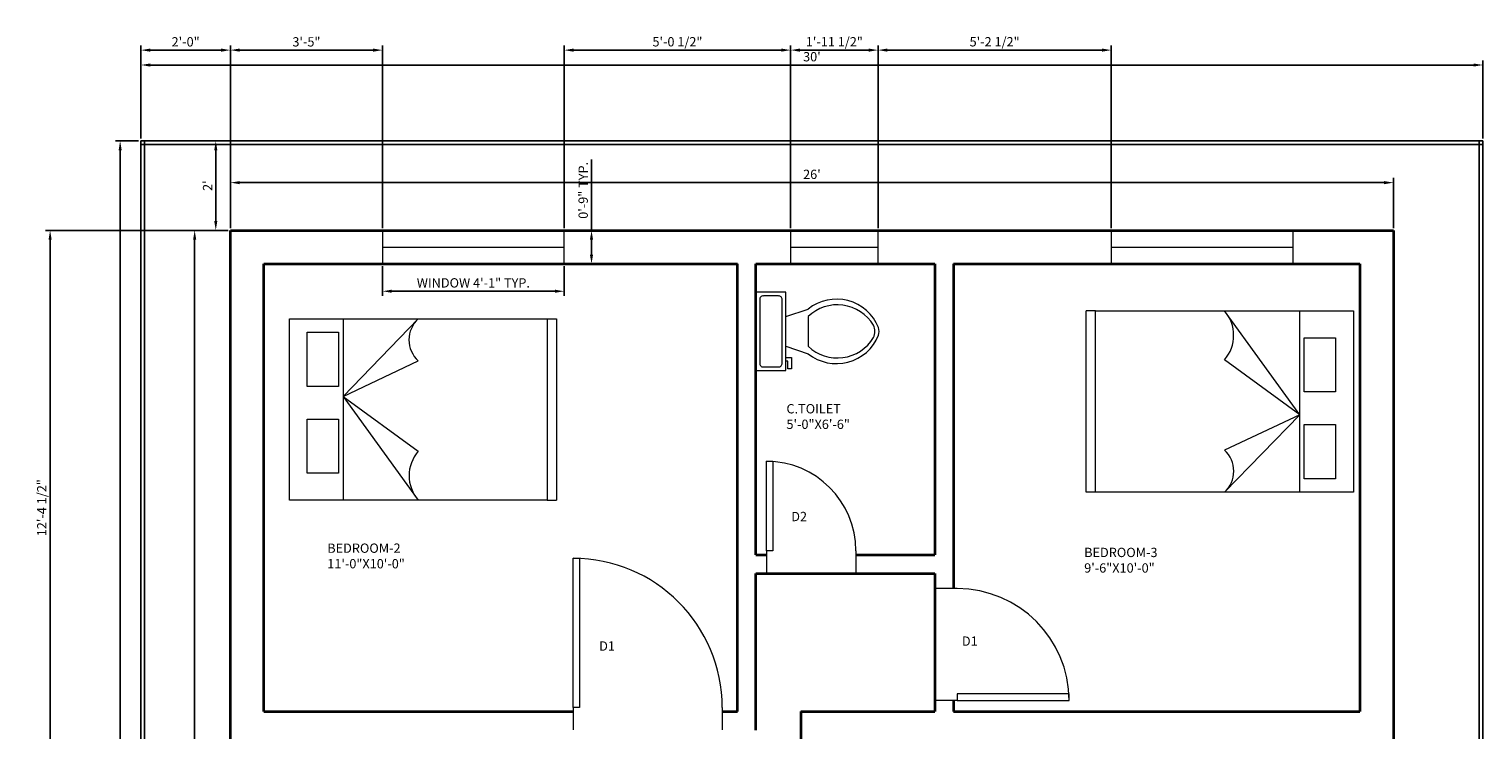
# Model space of a CAD drawing. Units: inches. Extents: x 0 to 3634, y 1847 to 2359.
# Tile 3 of 3: x 3218 to 3608, y 2171 to 2359. Entities that reach past the tile are written whole.
import ezdxf

# ---------------------------------------------------------------- set-up
doc = ezdxf.new("R2010")
doc.units = ezdxf.units.IN
for name, color, linetype, lineweight, true_color in [('A-ANNO-DIMS', 215, 'Continuous', 18, 0xa953a0), ('A-ANNO-TEXT', 215, 'Continuous', 18, 0xa953a0), ('A-AREA-IDEN', 9, 'Continuous', 18, 0xafd9aa), ('A-FURN', 254, 'Continuous', 18, 0xd7ebd2), ('A-GLAZ', 9, 'Continuous', 18, 0xafd9aa), ('C-PROP', 9, 'Continuous', 25, 0xafd9aa)]:
    doc.layers.add(name, color=color, linetype=linetype, lineweight=lineweight, true_color=true_color)
for name, color, linetype, lineweight in [('A-DOOR', 4, 'Continuous', 18), ('A-FLOR-FIXT', 9, 'Continuous', 18), ('A-WALL', 7, 'Continuous', 35)]:
    doc.layers.add(name, color=color, linetype=linetype, lineweight=lineweight)
doc.styles.get("Standard").update_dxf_attribs({"font": 'arial.ttf'})
doc.dimstyles.new('ISO-25', dxfattribs={"dimtxt": 2.5, "dimasz": 2.5, "dimexe": 1.25, "dimexo": 0.625, "dimtad": 1, "dimlunit": 3, "dimtxsty": 'Standard', "dimcen": 2.5, "dimadec": 0, "dimazin": 0, "dimtfac": 1, "dimtmove": 0, "dimatfit": 3, "dimfxl": 1, "dimarcsym": 0})

# ---------------------------------------------------------------- blocks, each defined once
blk = doc.blocks.new('*U5')
for p, q in [((9.5, -6), (9.5, -2)), ((-10, -8.5), (-8, -8.5)), ((-10, -9.5), (-10, -8.5)), ((-7, -9.5), (-10, -9.5)), ((-8, -8.5), (-8, -8)), ((-7, -8), (-7, -9.5)), ((-4, -8), (-6, -14)), ((4, -8), (6, -14)), ((4, -14), (-4, -14))]:
    blk.add_line(p, q)
blk.add_lwpolyline([(10.5, -8), (10.5, 0), (-10.5, 0), (-10.5, -8)], close=True)
for points in [[(-9.5, -2), (-9.5, -6)], [(8.5, -1), (-8.5, -1)], [(-8.5, -7), (8.5, -7)]]:
    blk.add_lwpolyline(points)
for centre, radius, start, end in [((-8.62, -1.88), 0.884, 81.8699, 188.1301), ((8.62, -1.88), 0.884, 351.8699, 98.1301), ((-8.62, -6.12), 0.884, 171.8699, 278.1301), ((8.62, -6.12), 0.884, 261.8699, 8.1301), ((3.52, -21.58), 12.17, 141.4691, 247.9714), ((4.2, -21.82), 11.33, 136.3677, 238.9468), ((-3.52, -21.58), 12.17, 292.0284, 38.5307), ((-4.2, -21.82), 11.33, 301.053, 43.6321), ((0, -27.88), 4, 245.7318, 294.2682), ((0, -29), 4, 254.8605, 285.1395)]:
    blk.add_arc(centre, radius, start, end)
blk = doc.blocks.new('*U7')
for p, q in [((0, 0), (0, -6)), ((40, 0), (40, -6))]:
    blk.add_line(p, q)
blk.add_lwpolyline([(0, 0), (0, 40), (1.75, 40), (1.75, 0)], close=True)
blk.add_arc((0, 0), 40, 0, 90)
blk = doc.blocks.new('*U9')
for p, q in [((0, 0), (0, -6)), ((24, 0), (24, -6))]:
    blk.add_line(p, q)
blk.add_lwpolyline([(0, 0), (0, 24), (1.75, 24), (1.75, 0)], close=True)
blk.add_arc((0, 0), 24, 0, 90)
blk = doc.blocks.new('*U8')
for p, q in [((-30, 0), (-30, -6)), ((0, 0), (0, -6))]:
    blk.add_line(p, q)
blk.add_lwpolyline([(0, 0), (0, 30), (-1.75, 30), (-1.75, 0)], close=True)
blk.add_arc((0, 0), 30, 90, 180)
blk = doc.blocks.new('*D11')
at = {"layer": 'A-ANNO-DIMS', "color": 0, "lineweight": -2, "transparency": 16777216}
for p, q in [((3271.39, 2329.31), (3266.86, 2329.31)), ((3268.11, 2307.81), (3268.11, 2326.81)), ((3271.39, 2305.31), (3266.86, 2305.31))]:
    blk.add_line(p, q, dxfattribs=at)
at = {"layer": 'A-ANNO-DIMS', "color": 0, "transparency": 16777216}
for points in [[(3267.69, 2326.81), (3268.52, 2326.81), (3268.11, 2329.31)], [(3267.69, 2307.81), (3268.52, 2307.81), (3268.11, 2305.31)]]:
    blk.add_solid(points, dxfattribs=at)
at = {"layer": 'Defpoints', "color": 0, "transparency": 16777216}
for p in [(3268.11, 2329.31), (3272.02, 2329.31), (3272.02, 2305.31)]:
    blk.add_point(p, dxfattribs=at)
at = {"layer": 'A-ANNO-DIMS', "color": 0, "transparency": 16777216, "insert": (3266.23, 2317.31), "char_height": 2.5, "attachment_point": 5, "rotation": 90}
blk.add_mtext("2'", dxfattribs=at)
blk = doc.blocks.new('*D12')
at = {"layer": 'A-ANNO-DIMS', "color": 0, "lineweight": -2, "transparency": 16777216}
for p, q in [((3271.39, 2305.31), (3261.19, 2305.31)), ((3262.44, 2302.81), (3262.44, 1875.81)), ((3271.39, 1873.31), (3261.19, 1873.31))]:
    blk.add_line(p, q, dxfattribs=at)
at = {"layer": 'A-ANNO-DIMS', "color": 0, "transparency": 16777216}
for points in [[(3262.03, 2302.81), (3262.86, 2302.81), (3262.44, 2305.31)], [(3262.03, 1875.81), (3262.86, 1875.81), (3262.44, 1873.31)]]:
    blk.add_solid(points, dxfattribs=at)
at = {"layer": 'Defpoints', "color": 0, "transparency": 16777216}
for p in [(3272.02, 2305.31), (3262.44, 1873.31), (3272.02, 1873.31)]:
    blk.add_point(p, dxfattribs=at)
at = {"layer": 'A-ANNO-DIMS', "color": 0, "transparency": 16777216, "insert": (3260.54, 2089.31), "char_height": 2.5, "attachment_point": 5, "rotation": 90}
blk.add_mtext("36'", dxfattribs=at)
blk = doc.blocks.new('*D13')
at = {"layer": 'A-ANNO-DIMS', "color": 0, "lineweight": -2, "transparency": 16777216}
for p, q in [((3272.02, 2305.93), (3272.02, 2319.37)), ((3274.52, 2318.12), (3581.52, 2318.12)), ((3584.02, 2305.93), (3584.02, 2319.37))]:
    blk.add_line(p, q, dxfattribs=at)
at = {"layer": 'A-ANNO-DIMS', "color": 0, "transparency": 16777216}
for points in [[(3274.52, 2318.53), (3274.52, 2317.7), (3272.02, 2318.12)], [(3581.52, 2318.53), (3581.52, 2317.7), (3584.02, 2318.12)]]:
    blk.add_solid(points, dxfattribs=at)
at = {"layer": 'Defpoints', "color": 0, "transparency": 16777216}
for p in [(3584.02, 2318.12), (3272.02, 2305.31), (3584.02, 2305.31)]:
    blk.add_point(p, dxfattribs=at)
at = {"layer": 'A-ANNO-DIMS', "color": 0, "transparency": 16777216, "insert": (3428.02, 2320.02), "char_height": 2.5, "attachment_point": 5}
blk.add_mtext("26'", dxfattribs=at)
blk = doc.blocks.new('*D14')
at = {"layer": 'A-ANNO-DIMS', "color": 0, "lineweight": -2, "transparency": 16777216}
for p, q in [((3248.02, 2329.93), (3248.02, 2350.92)), ((3250.52, 2349.67), (3605.52, 2349.67)), ((3608.02, 2329.93), (3608.02, 2350.92))]:
    blk.add_line(p, q, dxfattribs=at)
at = {"layer": 'A-ANNO-DIMS', "color": 0, "transparency": 16777216}
for points in [[(3250.52, 2350.08), (3250.52, 2349.25), (3248.02, 2349.67)], [(3605.52, 2350.08), (3605.52, 2349.25), (3608.02, 2349.67)]]:
    blk.add_solid(points, dxfattribs=at)
at = {"layer": 'Defpoints', "color": 0, "transparency": 16777216}
for p in [(3608.02, 2349.67), (3248.02, 2329.31), (3608.02, 2329.31)]:
    blk.add_point(p, dxfattribs=at)
at = {"layer": 'A-ANNO-DIMS', "color": 0, "transparency": 16777216, "insert": (3428.02, 2351.57), "char_height": 2.5, "attachment_point": 5}
blk.add_mtext("30'", dxfattribs=at)
blk = doc.blocks.new('*D15')
at = {"layer": 'A-ANNO-DIMS', "color": 0, "lineweight": -2, "transparency": 16777216}
for p, q in [((3247.39, 2329.31), (3241.2, 2329.31)), ((3242.45, 1875.81), (3242.45, 2326.81)), ((3247.39, 1873.31), (3241.2, 1873.31))]:
    blk.add_line(p, q, dxfattribs=at)
at = {"layer": 'A-ANNO-DIMS', "color": 0, "transparency": 16777216}
for points in [[(3242.04, 2326.81), (3242.87, 2326.81), (3242.45, 2329.31)], [(3242.04, 1875.81), (3242.87, 1875.81), (3242.45, 1873.31)]]:
    blk.add_solid(points, dxfattribs=at)
at = {"layer": 'Defpoints', "color": 0, "transparency": 16777216}
for p in [(3242.45, 2329.31), (3248.02, 2329.31), (3248.02, 1873.31)]:
    blk.add_point(p, dxfattribs=at)
at = {"layer": 'A-ANNO-DIMS', "color": 0, "transparency": 16777216, "insert": (3240.55, 2101.31), "char_height": 2.5, "attachment_point": 5, "rotation": 90}
blk.add_mtext("38'", dxfattribs=at)
blk = doc.blocks.new('BED-DOUBLE')
for p, q in [((14.39, 48.64), (14.39, 0)), ((34.57, 48.64), (14.39, 27.87)), ((69.14, 48.64), (71.68, 48.64)), ((71.68, 48.64), (71.68, 0)), ((14.39, 27.87), (34.57, 37.39)), ((14.39, 27.87), (34.57, 0)), ((14.39, 27.87), (34.57, 13.18)), ((69.14, 0), (71.68, 0))]:
    blk.add_line(p, q)
for points in [[(0, 48.64), (69.14, 48.64), (69.14, 0), (0, 0)], [(4.78, 45.09), (13.17, 45.09), (13.17, 30.55), (4.78, 30.55)], [(4.78, 21.77), (13.17, 21.77), (13.17, 7.23), (4.78, 7.23)]]:
    blk.add_lwpolyline(points, close=True)
for centre, radius, start, end in [((39.66, 43.02), 7.59, 132.1054, 227.8946), ((42.17, 6.59), 10.06, 139.0804, 220.9196)]:
    blk.add_arc(centre, radius, start, end)
blk = doc.blocks.new('WIN-48_77')
for p, q in [((0, 9), (0, 0)), ((48.77, 9), (0, 9)), ((0, 9), (0, 4.5)), ((48.77, 0), (48.77, 9)), ((0, 4.5), (48.77, 4.5)), ((0, 0), (48.77, 0))]:
    blk.add_line(p, q)
blk = doc.blocks.new('*D22')
at = {"layer": 'A-ANNO-DIMS', "color": 0, "lineweight": -2, "transparency": 16777216}
for p, q in [((3312.81, 2295.68), (3312.81, 2287.74)), ((3361.58, 2295.68), (3361.58, 2287.74)), ((3315.31, 2288.99), (3359.08, 2288.99))]:
    blk.add_line(p, q, dxfattribs=at)
at = {"layer": 'A-ANNO-DIMS', "color": 0, "transparency": 16777216}
for points in [[(3315.31, 2289.41), (3315.31, 2288.58), (3312.81, 2288.99)], [(3359.08, 2289.41), (3359.08, 2288.58), (3361.58, 2288.99)]]:
    blk.add_solid(points, dxfattribs=at)
at = {"layer": 'Defpoints', "color": 0, "transparency": 16777216}
for p in [(3312.81, 2296.31), (3361.58, 2296.31), (3361.58, 2288.99)]:
    blk.add_point(p, dxfattribs=at)
at = {"layer": 'A-ANNO-DIMS', "color": 0, "transparency": 16777216, "insert": (3337.2, 2290.91), "char_height": 2.5, "attachment_point": 5}
blk.add_mtext('WINDOW 4\'-1" TYP.', dxfattribs=at)
blk = doc.blocks.new('*D23')
at = {"layer": 'A-ANNO-DIMS', "color": 0, "lineweight": -2, "transparency": 16777216}
for p, q in [((3368.9, 2305.31), (3368.9, 2324.3)), ((3362.21, 2305.31), (3370.15, 2305.31)), ((3368.9, 2298.81), (3368.9, 2302.81)), ((3362.21, 2296.31), (3370.15, 2296.31))]:
    blk.add_line(p, q, dxfattribs=at)
at = {"layer": 'A-ANNO-DIMS', "color": 0, "transparency": 16777216}
for points in [[(3368.48, 2302.81), (3369.31, 2302.81), (3368.9, 2305.31)], [(3368.48, 2298.81), (3369.31, 2298.81), (3368.9, 2296.31)]]:
    blk.add_solid(points, dxfattribs=at)
at = {"layer": 'Defpoints', "color": 0, "transparency": 16777216}
for p in [(3361.58, 2305.31), (3368.9, 2305.31), (3361.58, 2296.31)]:
    blk.add_point(p, dxfattribs=at)
at = {"layer": 'A-ANNO-DIMS', "color": 0, "transparency": 16777216, "insert": (3366.99, 2316.05), "char_height": 2.5, "attachment_point": 5, "rotation": 90}
blk.add_mtext('0\'-9" TYP.', dxfattribs=at)
blk = doc.blocks.new('*D29')
at = {"layer": 'A-ANNO-DIMS', "color": 0, "lineweight": -2, "transparency": 16777216}
for p, q in [((3248.02, 2329.93), (3248.02, 2354.91)), ((3250.52, 2353.66), (3269.52, 2353.66)), ((3272.02, 2305.93), (3272.02, 2354.91))]:
    blk.add_line(p, q, dxfattribs=at)
at = {"layer": 'A-ANNO-DIMS', "color": 0, "transparency": 16777216}
for points in [[(3250.52, 2354.08), (3250.52, 2353.24), (3248.02, 2353.66)], [(3269.52, 2354.08), (3269.52, 2353.24), (3272.02, 2353.66)]]:
    blk.add_solid(points, dxfattribs=at)
at = {"layer": 'Defpoints', "color": 0, "transparency": 16777216}
for p in [(3272.02, 2353.66), (3248.02, 2329.31), (3272.02, 2305.31)]:
    blk.add_point(p, dxfattribs=at)
at = {"layer": 'A-ANNO-DIMS', "color": 0, "transparency": 16777216, "insert": (3260.02, 2355.56), "char_height": 2.5, "attachment_point": 5}
blk.add_mtext('2\'-0"', dxfattribs=at)
blk = doc.blocks.new('*D30')
at = {"layer": 'A-ANNO-DIMS', "color": 0, "lineweight": -2, "transparency": 16777216}
for p, q in [((3272.02, 2305.93), (3272.02, 2354.91)), ((3274.52, 2353.66), (3310.31, 2353.66)), ((3312.81, 2305.93), (3312.81, 2354.91))]:
    blk.add_line(p, q, dxfattribs=at)
at = {"layer": 'A-ANNO-DIMS', "color": 0, "transparency": 16777216}
for points in [[(3274.52, 2354.08), (3274.52, 2353.24), (3272.02, 2353.66)], [(3310.31, 2354.08), (3310.31, 2353.24), (3312.81, 2353.66)]]:
    blk.add_solid(points, dxfattribs=at)
at = {"layer": 'Defpoints', "color": 0, "transparency": 16777216}
for p in [(3312.81, 2353.66), (3272.02, 2305.31), (3312.81, 2305.31)]:
    blk.add_point(p, dxfattribs=at)
at = {"layer": 'A-ANNO-DIMS', "color": 0, "transparency": 16777216, "insert": (3292.42, 2355.56), "char_height": 2.5, "attachment_point": 5}
blk.add_mtext('3\'-5"', dxfattribs=at)
blk = doc.blocks.new('*D31')
at = {"layer": 'A-ANNO-DIMS', "color": 0, "lineweight": -2, "transparency": 16777216}
for p, q in [((3422.31, 2305.93), (3422.31, 2354.91)), ((3424.81, 2353.66), (3443.25, 2353.66)), ((3445.75, 2305.93), (3445.75, 2354.91))]:
    blk.add_line(p, q, dxfattribs=at)
at = {"layer": 'A-ANNO-DIMS', "color": 0, "transparency": 16777216}
for points in [[(3424.81, 2354.08), (3424.81, 2353.24), (3422.31, 2353.66)], [(3443.25, 2354.08), (3443.25, 2353.24), (3445.75, 2353.66)]]:
    blk.add_solid(points, dxfattribs=at)
at = {"layer": 'Defpoints', "color": 0, "transparency": 16777216}
for p in [(3445.75, 2353.66), (3422.31, 2305.31), (3445.75, 2305.31)]:
    blk.add_point(p, dxfattribs=at)
at = {"layer": 'A-ANNO-DIMS', "color": 0, "transparency": 16777216, "insert": (3434.03, 2355.58), "char_height": 2.5, "attachment_point": 5}
blk.add_mtext('1\'-11 1/2"', dxfattribs=at)
blk = doc.blocks.new('*D32')
at = {"layer": 'A-ANNO-DIMS', "color": 0, "lineweight": -2, "transparency": 16777216}
for p, q in [((3361.58, 2305.93), (3361.58, 2354.91)), ((3364.08, 2353.66), (3419.81, 2353.66)), ((3422.31, 2305.93), (3422.31, 2354.91))]:
    blk.add_line(p, q, dxfattribs=at)
at = {"layer": 'A-ANNO-DIMS', "color": 0, "transparency": 16777216}
for points in [[(3364.08, 2354.08), (3364.08, 2353.24), (3361.58, 2353.66)], [(3419.81, 2354.08), (3419.81, 2353.24), (3422.31, 2353.66)]]:
    blk.add_solid(points, dxfattribs=at)
at = {"layer": 'Defpoints', "color": 0, "transparency": 16777216}
for p in [(3422.31, 2353.66), (3361.58, 2305.31), (3422.31, 2305.31)]:
    blk.add_point(p, dxfattribs=at)
at = {"layer": 'A-ANNO-DIMS', "color": 0, "transparency": 16777216, "insert": (3391.95, 2355.58), "char_height": 2.5, "attachment_point": 5}
blk.add_mtext('5\'-0 1/2"', dxfattribs=at)
blk = doc.blocks.new('*D33')
at = {"layer": 'A-ANNO-DIMS', "color": 0, "lineweight": -2, "transparency": 16777216}
for p, q in [((3445.75, 2305.93), (3445.75, 2354.91)), ((3448.25, 2353.66), (3505.82, 2353.66)), ((3508.32, 2305.93), (3508.32, 2354.91))]:
    blk.add_line(p, q, dxfattribs=at)
at = {"layer": 'A-ANNO-DIMS', "color": 0, "transparency": 16777216}
for points in [[(3448.25, 2354.08), (3448.25, 2353.24), (3445.75, 2353.66)], [(3505.82, 2354.08), (3505.82, 2353.24), (3508.32, 2353.66)]]:
    blk.add_solid(points, dxfattribs=at)
at = {"layer": 'Defpoints', "color": 0, "transparency": 16777216}
for p in [(3508.32, 2353.66), (3445.75, 2305.31), (3508.32, 2305.31)]:
    blk.add_point(p, dxfattribs=at)
at = {"layer": 'A-ANNO-DIMS', "color": 0, "transparency": 16777216, "insert": (3477.03, 2355.58), "char_height": 2.5, "attachment_point": 5}
blk.add_mtext('5\'-2 1/2"', dxfattribs=at)
blk = doc.blocks.new('*D37')
at = {"layer": 'A-ANNO-DIMS', "color": 0, "lineweight": -2, "transparency": 16777216}
for p, q in [((3271.39, 2305.31), (3222.42, 2305.31)), ((3223.67, 2159.06), (3223.67, 2302.81)), ((3271.39, 2156.56), (3222.42, 2156.56))]:
    blk.add_line(p, q, dxfattribs=at)
at = {"layer": 'A-ANNO-DIMS', "color": 0, "transparency": 16777216}
for points in [[(3223.25, 2302.81), (3224.09, 2302.81), (3223.67, 2305.31)], [(3223.25, 2159.06), (3224.09, 2159.06), (3223.67, 2156.56)]]:
    blk.add_solid(points, dxfattribs=at)
at = {"layer": 'Defpoints', "color": 0, "transparency": 16777216}
for p in [(3223.67, 2305.31), (3272.02, 2305.31), (3272.02, 2156.56)]:
    blk.add_point(p, dxfattribs=at)
at = {"layer": 'A-ANNO-DIMS', "color": 0, "transparency": 16777216, "insert": (3221.75, 2230.93), "char_height": 2.5, "attachment_point": 5, "rotation": 90}
blk.add_mtext('12\'-4 1/2"', dxfattribs=at)

msp = doc.modelspace()

# ---------------------------------------------------------------- linework, layer by layer
at = {"layer": 'A-GLAZ'}
for p, q in [((3422.31, 2305.309), (3422.31, 2296.309)), ((3445.753, 2305.309), (3422.31, 2305.309)), ((3422.31, 2305.309), (3422.31, 2300.809)), ((3445.753, 2296.309), (3445.753, 2305.309)), ((3422.31, 2300.809), (3445.753, 2300.809)), ((3422.31, 2296.309), (3445.753, 2296.309))]:
    msp.add_line(p, q, dxfattribs=at)
at = {"layer": 'A-WALL'}
for p, q in [((3272.018, 2305.309), (3584.018, 2305.309)), ((3272.018, 1873.309), (3272.018, 2305.309)), ((3584.018, 2305.309), (3584.018, 1873.309)), ((3281.018, 2296.309), (3408.018, 2296.309)), ((3281.018, 2176.309), (3281.018, 2296.309)), ((3408.018, 2176.309), (3408.018, 2296.309)), ((3413.018, 2218.309), (3413.018, 2296.309)), ((3413.018, 2296.309), (3461.018, 2296.309)), ((3461.018, 2296.309), (3461.018, 2218.309)), ((3466.018, 2296.309), (3466.018, 2209.223)), ((3466.018, 2296.309), (3575.018, 2296.309)), ((3575.018, 2296.309), (3575.018, 2176.309)), ((3413.018, 2218.309), (3415.798, 2218.309)), ((3439.798, 2218.309), (3461.018, 2218.309)), ((3413.018, 2213.309), (3461.018, 2213.309)), ((3413.018, 2171.309), (3413.018, 2213.309)), ((3461.018, 2213.309), (3461.018, 2176.309)), ((3281.018, 2176.309), (3363.96, 2176.309)), ((3403.96, 2176.309), (3408.018, 2176.309)), ((3425.018, 2176.309), (3461.018, 2176.309)), ((3425.018, 2176.309), (3425.018, 2120.548)), ((3466.018, 2179.223), (3466.018, 2176.309)), ((3466.018, 2176.309), (3575.018, 2176.309))]:
    msp.add_line(p, q, dxfattribs=at)
at = {"layer": 'C-PROP'}
for p, q in [((3272.018, 2329.309), (3248.018, 2329.309)), ((3248.018, 2329.309), (3248.018, 1873.309)), ((3272.018, 2328.309), (3248.018, 2328.309)), ((3249.018, 2329.309), (3249.018, 1873.309)), ((3272.018, 2329.309), (3608.018, 2329.309)), ((3272.018, 2328.309), (3608.018, 2328.309)), ((3607.018, 2329.309), (3607.018, 2305.309)), ((3608.018, 2329.309), (3608.018, 2305.309)), ((3607.018, 2305.309), (3607.018, 1873.309)), ((3608.018, 2305.309), (3608.018, 1873.309))]:
    msp.add_line(p, q, dxfattribs=at)

# ---------------------------------------------------------------- block references
at = {"layer": 'A-DOOR'}
for name, p in [('*U9', (3415.798, 2219.379)), ('*U7', (3363.96, 2177.356))]:
    msp.add_blockref(name, p, dxfattribs=at)
at = {"layer": 'A-DOOR', "rotation": 270}
msp.add_blockref('*U8', (3467.009, 2179.223), dxfattribs=at)
at = {"layer": 'A-FLOR-FIXT', "rotation": 89.99999999999935}
msp.add_blockref('*U5', (3413.018, 2278.218), dxfattribs=at)
at = {"layer": 'A-FURN'}
msp.add_blockref('BED-DOUBLE', (3287.852, 2232.929), dxfattribs=at)
at = {"layer": 'A-FURN', "rotation": 180}
msp.add_blockref('BED-DOUBLE', (3573.259, 2283.755), dxfattribs=at)
at = {"layer": 'A-GLAZ'}
for p in [(3312.813, 2296.309), (3508.317, 2296.309)]:
    msp.add_blockref('WIN-48_77', p, dxfattribs=at)

# ---------------------------------------------------------------- texts
at = {"layer": 'A-ANNO-TEXT', "char_height": 2.5, "attachment_point": 1}
for s, width, insert in [('D2', 12.1887, (3422.468, 2229.811)), ('D1', 13.52649, (3468.25, 2196.401)), ('D1', 18.22108, (3370.949, 2195.086))]:
    msp.add_mtext_dynamic_manual_height_columns(s, width=width, gutter_width=12.5, heights=[0], dxfattribs=dict(at, insert=insert))
at = {"layer": 'A-AREA-IDEN', "char_height": 2.5, "attachment_point": 1}
for s, width, insert in [('C.TOILET\\P5\'-0"X6\'-6"', 23.79242, (3421.187, 2258.723)), ('BEDROOM-2\\P11\'-0"X10\'-0"', 45.12201, (3298.013, 2221.329)), ('BEDROOM-3\\P9\'-6"X10\'-0"', 42.01738, (3501.056, 2220.188))]:
    msp.add_mtext_dynamic_manual_height_columns(s, width=width, gutter_width=12.5, heights=[0], dxfattribs=dict(at, insert=insert))

# ---------------------------------------------------------------- dimensions: what is measured, and where the dimension line sits
at = {"layer": 'A-ANNO-DIMS'}
for base, p1, p2, override, picture, middle in [((3272.018, 2353.659), (3248.018, 2329.309), (3272.018, 2305.309), {"dimdec": 1, "dimlfac": 1, "dimrnd": 0, "dimzin": 1, "dimdsep": 46, "dimlunit": 4, "dimfrac": 2}, '*D29', (3260.018, 2355.56)), ((3312.813, 2353.659), (3272.018, 2305.309), (3312.813, 2305.309), {"dimdec": 1, "dimlfac": 1, "dimrnd": 0, "dimzin": 1, "dimdsep": 46, "dimlunit": 4, "dimfrac": 2}, '*D30', (3292.415, 2355.561)), ((3422.31, 2353.659), (3361.58, 2305.309), (3422.31, 2305.309), {"dimdec": 1, "dimlfac": 1, "dimrnd": 0, "dimzin": 1, "dimdsep": 46, "dimlunit": 4, "dimfrac": 2}, '*D32', (3391.945, 2355.577)), ((3445.753, 2353.659), (3422.31, 2305.309), (3445.753, 2305.309), {"dimdec": 1, "dimlfac": 1, "dimrnd": 0, "dimzin": 1, "dimdsep": 46, "dimlunit": 4, "dimfrac": 2}, '*D31', (3434.032, 2355.577)), ((3508.317, 2353.659), (3445.753, 2305.309), (3508.317, 2305.309), {"dimdec": 1, "dimlfac": 1, "dimrnd": 0, "dimzin": 1, "dimdsep": 46, "dimlunit": 4, "dimfrac": 2}, '*D33', (3477.035, 2355.577)), ((3608.018, 2349.667), (3248.018, 2329.309), (3608.018, 2329.309), {"dimclrd": 0, "dimclre": 0, "dimclrt": 0}, '*D14', (3428.018, 2351.569)), ((3584.018, 2318.117), (3272.018, 2305.309), (3584.018, 2305.309), {"dimclrd": 0, "dimclre": 0, "dimclrt": 0}, '*D13', (3428.018, 2320.018))]:
    dim = msp.add_linear_dim(base=base, p1=p1, p2=p2, dimstyle='ISO-25', override=override, dxfattribs=at)
    dim.commit()
    dim.dimension.update_dxf_attribs({"geometry": picture, "text_midpoint": middle})
for base, p1, p2, override, picture, middle in [((3242.454, 2329.309), (3248.018, 1873.309), (3248.018, 2329.309), {"dimclrd": 0, "dimclre": 0, "dimclrt": 0}, '*D15', (3240.552, 2101.309)), ((3268.107, 2329.309), (3272.018, 2305.309), (3272.018, 2329.309), {"dimclrd": 0, "dimclre": 0, "dimclrt": 0}, '*D11', (3266.226, 2317.309)), ((3223.668, 2305.309), (3272.018, 2156.56), (3272.018, 2305.309), {"dimdec": 1, "dimlfac": 1, "dimrnd": 0, "dimzin": 1, "dimdsep": 46, "dimlunit": 4, "dimfrac": 2}, '*D37', (3221.751, 2230.934)), ((3262.442, 1873.309), (3272.018, 2305.309), (3272.018, 1873.309), {"dimclrd": 0, "dimclre": 0, "dimclrt": 0}, '*D12', (3260.54, 2089.309))]:
    dim = msp.add_linear_dim(base=base, p1=p1, p2=p2, angle=90, dimstyle='ISO-25', override=override, dxfattribs=at)
    dim.commit()
    dim.dimension.update_dxf_attribs({"geometry": picture, "text_midpoint": middle})
dim = msp.add_linear_dim(base=(3368.895, 2305.309), p1=(3361.58, 2296.309), p2=(3361.58, 2305.309), angle=90, text='<> TYP.', dimstyle='ISO-25', override={"dimdec": 1, "dimlfac": 1, "dimrnd": 0, "dimzin": 1, "dimdsep": 46, "dimlunit": 4, "dimfrac": 2}, dxfattribs=at)
dim.commit()
dim.dimension.update_dxf_attribs({"geometry": '*D23', "text_midpoint": (3366.994, 2316.053)})
dim = msp.add_linear_dim(base=(3361.58, 2288.994), p1=(3312.813, 2296.309), p2=(3361.58, 2296.309), text='WINDOW <> TYP.', dimstyle='ISO-25', override={"dimdec": 1, "dimlfac": 1, "dimrnd": 0, "dimzin": 1, "dimdsep": 46, "dimlunit": 4, "dimfrac": 2}, dxfattribs=at)
dim.commit()
dim.dimension.update_dxf_attribs({"geometry": '*D22', "text_midpoint": (3337.196, 2290.912)})

doc.saveas('drawing.dxf')
